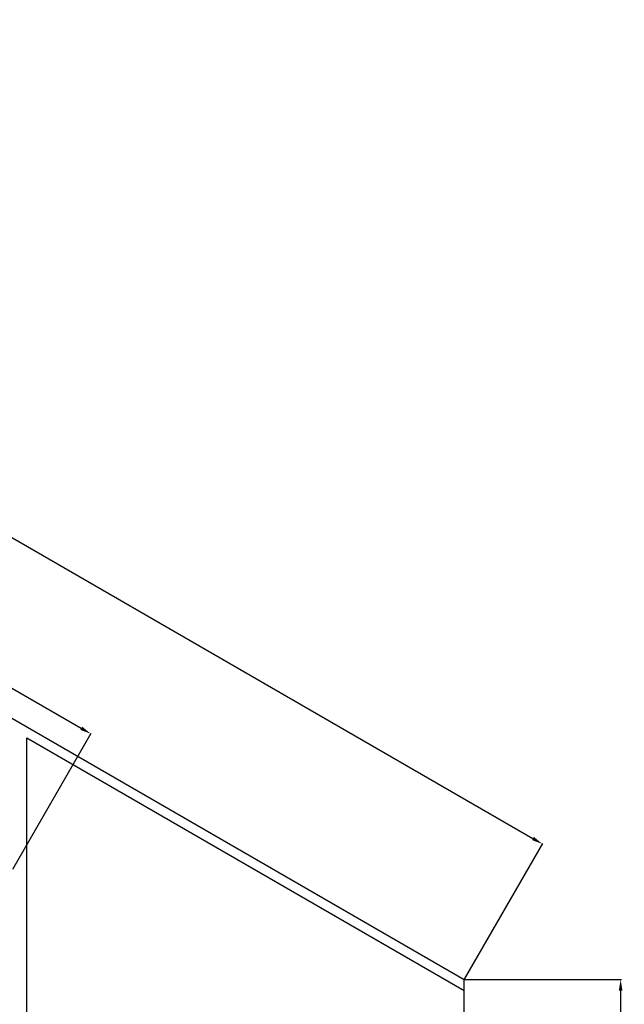
# Model space of a CAD drawing. Units: centimetres. Extents: x 209356 to 217348, y 253987 to 259034.
# Tile 7 of 7: x 214078 to 215179, y 257241 to 259034. Entities that reach past the tile are written whole.
import ezdxf

# ---------------------------------------------------------------- set-up
doc = ezdxf.new("R2010")
doc.units = ezdxf.units.CM
doc.layers.add('A-ANNO-DIMS', color=2, linetype='Continuous', lineweight=18)
doc.layers.add('A-ELEV', color=7, linetype='Continuous', lineweight=25)
doc.styles.get("Standard").update_dxf_attribs({"font": 'arial.ttf'})
doc.dimstyles.new('ISO-25', dxfattribs={"dimtxt": 50, "dimasz": 20, "dimexe": 1.25, "dimexo": 0.625, "dimtad": 1, "dimdec": 1, "dimtxsty": 'Standard', "dimcen": 2.5, "dimadec": 0, "dimazin": 0, "dimtfac": 1, "dimtdec": 1, "dimtmove": 0, "dimatfit": 3, "dimfxl": 1, "dimarcsym": 0})

# ---------------------------------------------------------------- blocks, each defined once
blk = doc.blocks.new('*D10')
at = {"layer": 'A-ANNO-DIMS', "color": 0, "lineweight": -2, "transparency": 16777216}
for p, q in [((212289.9, 258787.1), (212432.7, 259034.4)), ((212449.4, 259023.4), (215012.8, 257543.4)), ((214888, 257287.1), (215030.8, 257534.4))]:
    blk.add_line(p, q, dxfattribs=at)
at = {"layer": 'A-ANNO-DIMS', "color": 0, "transparency": 16777216}
for points in [[(212451.1, 259026.3), (212447.7, 259020.5), (212432.1, 259033.4)], [(215014.5, 257546.3), (215011.2, 257540.5), (215030.1, 257533.4)]]:
    blk.add_solid(points, dxfattribs=at)
at = {"layer": 'Defpoints', "color": 0, "transparency": 16777216}
for p in [(212289.6, 258786.5), (215030.1, 257533.4), (214887.6, 257286.5)]:
    blk.add_point(p, dxfattribs=at)
at = {"layer": 'A-ANNO-DIMS', "color": 0, "transparency": 16777216, "insert": (213744.2, 258306), "char_height": 50, "attachment_point": 5, "rotation": 330}
blk.add_mtext('3000', dxfattribs=at)
blk = doc.blocks.new('*D11')
at = {"layer": 'A-ANNO-DIMS', "color": 0, "lineweight": -2, "transparency": 16777216}
for p, q in [((214888.3, 257286.5), (215173.9, 257286.5)), ((215172.6, 257266.5), (215172.6, 254886.5)), ((214888.3, 254866.5), (215173.9, 254866.5))]:
    blk.add_line(p, q, dxfattribs=at)
at = {"layer": 'A-ANNO-DIMS', "color": 0, "transparency": 16777216}
for points in [[(215169.3, 257266.5), (215176, 257266.5), (215172.6, 257286.5)], [(215169.3, 254886.5), (215176, 254886.5), (215172.6, 254866.5)]]:
    blk.add_solid(points, dxfattribs=at)
at = {"layer": 'Defpoints', "color": 0, "transparency": 16777216}
for p in [(214887.6, 257286.5), (214887.6, 254866.5), (215172.6, 254866.5)]:
    blk.add_point(p, dxfattribs=at)
at = {"layer": 'A-ANNO-DIMS', "color": 0, "transparency": 16777216, "insert": (215146.5, 256076.5), "char_height": 50, "attachment_point": 5, "rotation": 90}
blk.add_mtext('2420', dxfattribs=at)
blk = doc.blocks.new('*D22')
at = {"layer": 'A-ANNO-DIMS', "color": 0, "lineweight": -2, "transparency": 16777216}
for p, q in [((213157.7, 258011.7), (213300.5, 258259.1)), ((213317.2, 258248), (214190.1, 257744.1)), ((214065.2, 257487.8), (214208, 257735.2))]:
    blk.add_line(p, q, dxfattribs=at)
at = {"layer": 'A-ANNO-DIMS', "color": 0, "transparency": 16777216}
for points in [[(213318.9, 258250.9), (213315.6, 258245.1), (213299.9, 258258)], [(214191.8, 257747), (214188.4, 257741.2), (214207.4, 257734.1)]]:
    blk.add_solid(points, dxfattribs=at)
at = {"layer": 'Defpoints', "color": 0, "transparency": 16777216}
for p in [(213157.4, 258011.2), (214207.4, 257734.1), (214064.9, 257487.3)]:
    blk.add_point(p, dxfattribs=at)
at = {"layer": 'A-ANNO-DIMS', "color": 0, "transparency": 16777216, "insert": (213766.7, 258018.7), "char_height": 50, "attachment_point": 5, "rotation": 330}
blk.add_mtext('1047.9', dxfattribs=at)

msp = doc.modelspace()

# ---------------------------------------------------------------- linework, layer by layer
at = {"layer": 'A-ELEV'}
for p, q in [((212289.5688, 258786.5492), (214887.645, 257286.5492)), ((214090.9016, 255326.5492), (214090.9016, 257726.5492)), ((214090.9016, 257726.5492), (214887.645, 257266.5492)), ((214887.645, 254846.5492), (214887.645, 257286.5492))]:
    msp.add_line(p, q, dxfattribs=at)

# ---------------------------------------------------------------- dimensions: what is measured, and where the dimension line sits
at = {"layer": 'A-ANNO-DIMS'}
for base, p1, p2, angle, override, picture, middle in [((215030.145, 257533.3664), (212289.5688, 258786.5492), (214887.645, 257286.5492), 330, {"dimdec": 0, "dimlfac": 1, "dimrnd": 0, "dimzin": 0, "dimdsep": 46, "dimlunit": 2}, '*D10', (213744.1922, 258306.0309)), ((214207.4209, 257734.0709), (213157.4217, 258011.1985), (214064.9209, 257487.2537), 330, {"dimdec": 1, "dimlfac": 1, "dimrnd": 0, "dimzin": 0, "dimdsep": 46, "dimlunit": 2}, '*D22', (213766.7481, 258018.6931)), ((215172.645, 254866.5492), (214887.645, 257286.5492), (214887.645, 254866.5492), 270, {"dimdec": 0, "dimlfac": 1, "dimrnd": 0, "dimzin": 0, "dimdsep": 46, "dimlunit": 2}, '*D11', (215146.4913, 256076.5492))]:
    dim = msp.add_linear_dim(base=base, p1=p1, p2=p2, angle=angle, dimstyle='ISO-25', override=override, dxfattribs=at)
    dim.commit()
    dim.dimension.update_dxf_attribs({"geometry": picture, "text_midpoint": middle})

doc.saveas('drawing.dxf')
